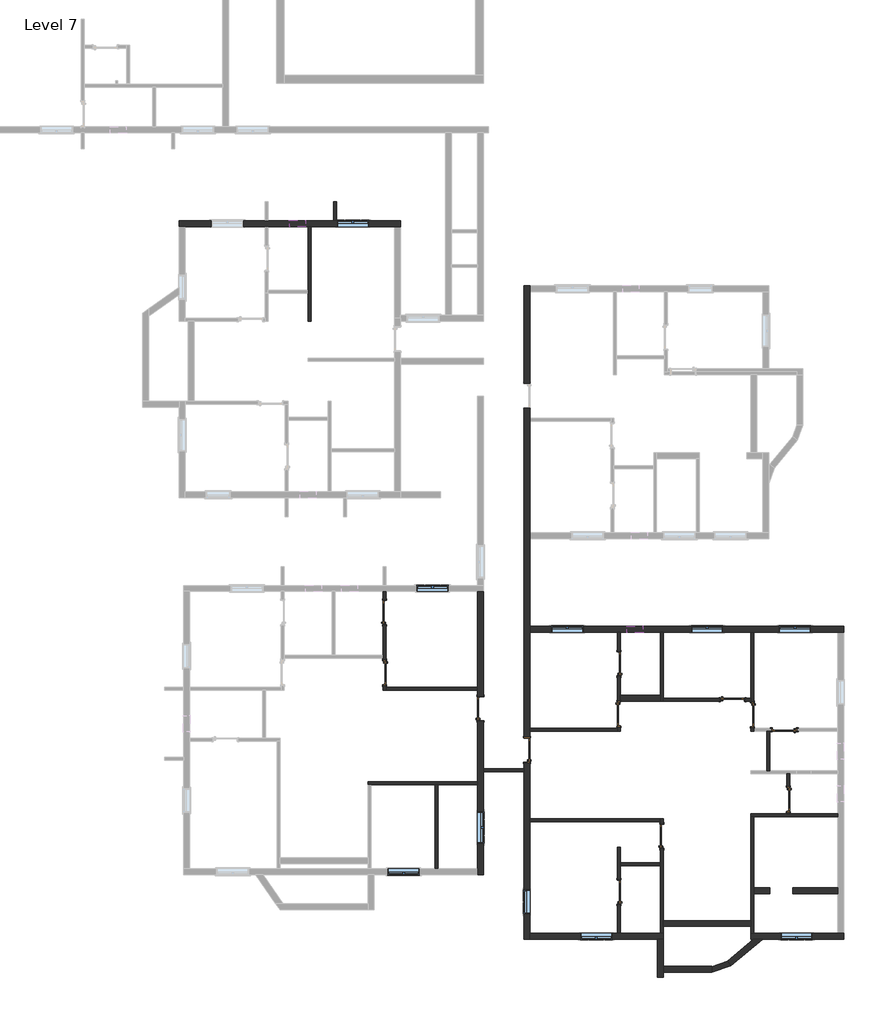
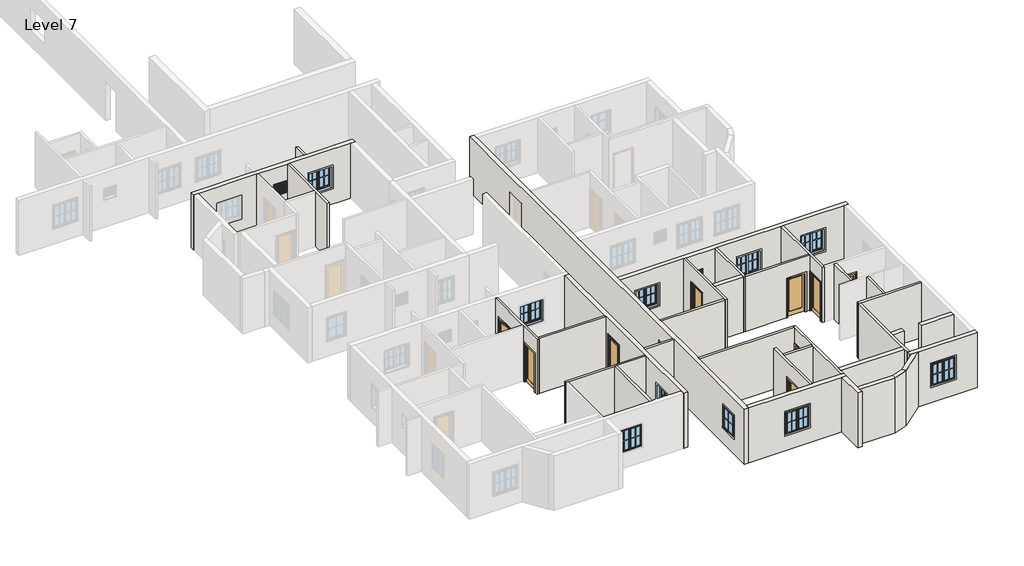
# One storey, part 2 of 7: 34 walls, 12 doors, 12 windows.
# Revit data of these elements (continued)
# Element 48 (IfcWindow, "Window-Casement-Double : 4' x 4'") (continued)
#   Materials on its faces: "Wood - Stained", "Glass", "Clad - White"
# Element 49 (IfcWindow, "Window-Casement-Double : 4' x 4'")
#   Mark = "178"
#   Window Inset = 0' - 0"
#   Interior Wall Closure = 0' - 2 1/4"
#   Frame Extension = 0' - 0 1/4"
#   Exterior Wall Closure = 0' - 1 1/4"
#   Interior Trim Visibility = yes
#   Exterior Trim Visibility = yes
#   Phase Created = New Construction
#   Materials on its faces: "Wood - Stained", "Glass", "Clad - White"
# Element 50 (IfcWindow, "Window-Casement-Double : 4' x 4'")
#   Mark = "179"
#   Window Inset = 0' - 0"
#   Interior Wall Closure = 0' - 2 1/4"
#   Frame Extension = 0' - 0 1/4"
#   Exterior Wall Closure = 0' - 1 1/4"
#   Interior Trim Visibility = yes
#   Exterior Trim Visibility = yes
#   Phase Created = New Construction
#   Materials on its faces: "Wood - Stained", "Glass", "Clad - White"
# Element 51 (IfcWindow, "Window-Casement-Double : 4' x 4'")
#   Mark = "180"
#   Window Inset = 0' - 0"
#   Interior Wall Closure = 0' - 2 1/4"
#   Frame Extension = 0' - 0 1/4"
#   Exterior Wall Closure = 0' - 1 1/4"
#   Interior Trim Visibility = yes
#   Exterior Trim Visibility = yes
#   Phase Created = New Construction
#   Materials on its faces: "Wood - Stained", "Glass", "Clad - White"
# Element 52 (IfcWindow, "Window-Casement-Double : 4' x 4'")
#   Mark = "181"
#   Window Inset = 0' - 0"
#   Interior Wall Closure = 0' - 2 1/4"
#   Frame Extension = 0' - 0 1/4"
#   Exterior Wall Closure = 0' - 1 1/4"
#   Interior Trim Visibility = yes
#   Exterior Trim Visibility = yes
#   Phase Created = New Construction
#   Materials on its faces: "Wood - Stained", "Glass", "Clad - White"
# Element 53 (IfcWindow, "Window-Casement-Double : 4' x 4'")
#   Mark = "182"
#   Window Inset = 0' - 0"
#   Interior Wall Closure = 0' - 2 1/4"
#   Frame Extension = 0' - 0 1/4"
#   Exterior Wall Closure = 0' - 1 1/4"
#   Interior Trim Visibility = yes
#   Exterior Trim Visibility = yes
#   Phase Created = New Construction
#   Materials on its faces: "Wood - Stained", "Glass", "Clad - White"
# Element 54 (IfcWindow, "Window-Casement-Double : 4' x 4'")
#   Mark = "183"
#   Window Inset = 0' - 0"
#   Interior Wall Closure = 0' - 2 1/4"
#   Frame Extension = 0' - 0 1/4"
#   Exterior Wall Closure = 0' - 1 1/4"
#   Interior Trim Visibility = yes
#   Exterior Trim Visibility = yes
#   Phase Created = New Construction
#   Materials on its faces: "Wood - Stained", "Glass", "Clad - White"
# Element 55 (IfcWindow, "Window-Casement-Double : 4' x 4'")
#   Mark = "185"
#   Window Inset = 0' - 0"
#   Interior Wall Closure = 0' - 2 1/4"
#   Frame Extension = 0' - 0 1/4"
#   Exterior Wall Closure = 0' - 1 1/4"
#   Interior Trim Visibility = yes
#   Exterior Trim Visibility = yes
#   Phase Created = New Construction
#   Materials on its faces: "Wood - Stained", "Glass", "Clad - White"
# Element 56 (IfcWindow, "Window-Casement-Double : 4' x 4'")
#   Mark = "192"
#   Window Inset = 0' - 0"
#   Interior Wall Closure = 0' - 2 1/4"
#   Frame Extension = 0' - 0 1/4"
#   Exterior Wall Closure = 0' - 1 1/4"
#   Interior Trim Visibility = yes
#   Exterior Trim Visibility = yes
#   Phase Created = New Construction
#   Materials on its faces: "Wood - Stained", "Glass", "Clad - White"
# Element 57 (IfcWindow, "Window-Louvers : 24\" x 24\"")
#   Mark = "139"
#   Blade Width = 1' - 10 1/2"
#   Phase Created = New Construction
#   Materials on its faces: "Birch"
# Element 58 (IfcWindow, "Window-Louvers : 24\" x 24\"")
#   Mark = "145"
#   Blade Width = 1' - 10 1/2"
#   Phase Created = New Construction
#   Materials on its faces: "Birch"
# Materials
#   "Cherry": class "Wood", colour RGB 226 177 128, transparency 0, Description = "Prunus Serotina", Cost = 0
#   "Aluminum": class "Metal", colour RGB 247 247 247, transparency 0, Description = "Aluminum 6061", Cost = 0
#   "Wood - Stained": class "Wood", colour RGB 224 178 126, transparency 0, Cost = 0
#   "Glass": class "Glass", colour RGB 0 128 192, transparency 0.75, Description = "Soda Lime Glass", Cost = 0
#   "Clad - White": class "Wood", colour RGB 242 242 238, transparency 0, Cost = 0
#   "Birch": class "Wood", colour RGB 224 178 126, transparency 0, Description = "Betula Alleghaniensis", Cost = 0
#   "Default Wall": colour RGB 128 128 128, transparency 0, Cost = 0
